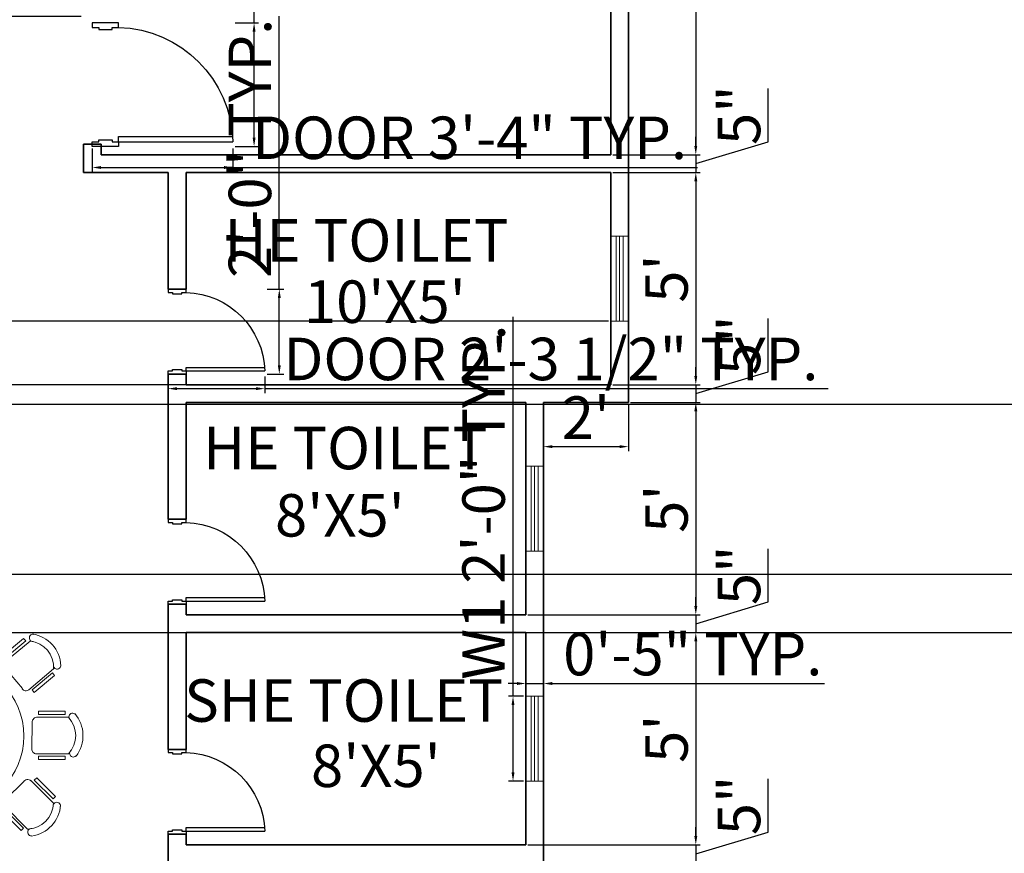
# Model space of a CAD drawing. Units: inches. Extents: x 2319 to 3765, y 2872 to 3950.
# Tile 6 of 9: x 2783 to 3061, y 3121 to 3357. Entities that reach past the tile are written whole.
import ezdxf

# ---------------------------------------------------------------- set-up
doc = ezdxf.new("R2010")
doc.units = ezdxf.units.IN
for name, color, linetype, lineweight in [('A-ANNO-DIMS', 2, 'Continuous', 18), ('A-AREA-IDEN', 7, 'Continuous', 18), ('A-DOOR', 3, 'Continuous', 25), ('A-FURN', 8, 'Continuous', 18), ('A-GLAZ', 4, 'Continuous', 18), ('A-WALL', 7, 'Continuous', 35)]:
    doc.layers.add(name, color=color, linetype=linetype, lineweight=lineweight)
doc.styles.get("Standard").update_dxf_attribs({"font": 'arial.ttf'})
doc.dimstyles.new('ISO-25', dxfattribs={"dimtxt": 12, "dimasz": 2.5, "dimexe": 1.25, "dimexo": 0.625, "dimtad": 1, "dimdec": 0, "dimlunit": 3, "dimtxsty": 'Standard', "dimcen": 2.5, "dimadec": 0, "dimazin": 0, "dimtfac": 1, "dimtdec": 0, "dimtmove": 0, "dimatfit": 3, "dimfxl": 1, "dimarcsym": 0})

# ---------------------------------------------------------------- blocks, each defined once
blk = doc.blocks.new('*D1')
at = {"layer": 'A-ANNO-DIMS', "color": 0, "lineweight": -2, "transparency": 16777216}
for p, q in [((2931.13, 3247.99), (2931.13, 3234.88)), ((2955.13, 3247.99), (2955.13, 3234.88)), ((2933.63, 3236.13), (2952.63, 3236.13))]:
    blk.add_line(p, q, dxfattribs=at)
at = {"layer": 'A-ANNO-DIMS', "color": 0, "transparency": 16777216}
for points in [[(2933.63, 3236.55), (2933.63, 3235.71), (2931.13, 3236.13)], [(2952.63, 3236.55), (2952.63, 3235.71), (2955.13, 3236.13)]]:
    blk.add_solid(points, dxfattribs=at)
at = {"layer": 'Defpoints', "color": 0, "transparency": 16777216}
for p in [(2931.13, 3248.61), (2955.13, 3248.61), (2955.13, 3236.13)]:
    blk.add_point(p, dxfattribs=at)
at = {"layer": 'A-ANNO-DIMS', "color": 0, "transparency": 16777216, "insert": (2943.13, 3242.78), "char_height": 12, "attachment_point": 5}
blk.add_mtext("2'", dxfattribs=at)
blk = doc.blocks.new('A$C769D55ED')
for p, q in [((33.6, 192), (33.6, 1024.8)), ((72, 192), (72, 1023.9)), ((0, 192), (0, 0)), ((33.6, 192), (0, 192)), ((33.6, 144), (33.6, 192)), ((48, 144), (33.6, 144)), ((48, 48), (48, 144)), ((33.6, 0), (33.6, 48)), ((33.6, 48), (48, 48)), ((0, 0), (33.6, 0))]:
    blk.add_line(p, q)
blk.add_lwpolyline([(33.6, 192), (72, 192)])
blk.add_lwpolyline([(900, 192), (900, 0), (866.4, 0), (866.4, 48), (852, 48), (852, 144), (866.4, 144), (866.4, 192)], close=True)
blk.add_arc((7.2, 165.6), 859.6, 1.76235, 88.23765)
blk = doc.blocks.new('A$C0EDB4AB9')
at = {"linetype": 'ByBlock'}
for p, q in [((1257, 3447), (1257, 3084)), ((1303, 3447), (1257, 3447)), ((1303, 3084), (1303, 3447)), ((1342, 3055), (1342, 3493)), ((1842, 3493), (1842, 3051)), ((1873, 3447), (1873, 3084)), ((1919, 3447), (1873, 3447)), ((1919, 3084), (1919, 3447)), ((2028, 3447), (2028, 3084)), ((2074, 3447), (2028, 3447)), ((2074, 3084), (2074, 3447)), ((2114, 3055), (2114, 3493)), ((2614, 3493), (2614, 3051)), ((2644, 3447), (2644, 3084)), ((2691, 3447), (2644, 3447)), ((2691, 3084), (2691, 3447)), ((2790, 3447), (2790, 3084)), ((2836, 3447), (2790, 3447)), ((2836, 3084), (2836, 3447)), ((2875, 3055), (2875, 3493)), ((3375, 3493), (3375, 3051)), ((3406, 3447), (3406, 3084)), ((3452, 3447), (3406, 3447)), ((3452, 3084), (3452, 3447)), ((3537, 3447), (3537, 3084)), ((3583, 3447), (3537, 3447)), ((3583, 3084), (3583, 3447)), ((3622, 3055), (3622, 3493)), ((4122, 3493), (4122, 3051)), ((4153, 3447), (4153, 3084)), ((4199, 3447), (4153, 3447)), ((4199, 3084), (4199, 3447)), ((4314, 3447), (4314, 3084)), ((4360, 3447), (4314, 3447)), ((4360, 3084), (4360, 3447)), ((4399, 3055), (4399, 3493)), ((4899, 3493), (4899, 3051)), ((4930, 3447), (4930, 3084)), ((4976, 3447), (4930, 3447)), ((4976, 3084), (4976, 3447)), ((5158, 3447), (5158, 3084)), ((5204, 3447), (5158, 3447)), ((5204, 3084), (5204, 3447)), ((5243, 3055), (5243, 3493)), ((5743, 3493), (5743, 3051)), ((5774, 3447), (5774, 3084)), ((5820, 3447), (5774, 3447)), ((5820, 3084), (5820, 3447)), ((5991, 3447), (5991, 3084)), ((6037, 3447), (5991, 3447)), ((6037, 3084), (6037, 3447)), ((6076, 3055), (6076, 3493)), ((6576, 3493), (6576, 3051)), ((6607, 3447), (6607, 3084)), ((6653, 3447), (6607, 3447)), ((6653, 3084), (6653, 3447)), ((770, 3117), (1098, 2820)), ((855, 3143), (824, 3109)), ((824, 3109), (1094, 2865)), ((1124, 2900), (855, 3143)), ((7050, 3209), (6772, 2975)), ((6802, 2940), (7080, 3173)), ((6804, 2891), (7139, 3172)), ((7080, 3173), (7050, 3209)), ((1257, 3084), (1303, 3084)), ((1772, 2993), (1413, 2995)), ((1791, 2993), (1772, 2993)), ((1873, 3084), (1919, 3084)), ((2028, 3084), (2074, 3084)), ((2544, 2993), (2185, 2995)), ((2562, 2993), (2544, 2993)), ((2644, 3084), (2691, 3084)), ((2790, 3084), (2836, 3084)), ((3305, 2993), (2946, 2995)), ((3324, 2993), (3305, 2993)), ((3406, 3084), (3452, 3084)), ((3537, 3084), (3583, 3084)), ((4052, 2993), (3693, 2995)), ((4070, 2993), (4052, 2993)), ((4153, 3084), (4199, 3084)), ((4314, 3084), (4360, 3084)), ((4829, 2993), (4470, 2995)), ((4847, 2993), (4829, 2993)), ((4930, 3084), (4976, 3084)), ((5158, 3084), (5204, 3084)), ((5673, 2993), (5314, 2995)), ((5692, 2993), (5673, 2993)), ((5774, 3084), (5820, 3084)), ((5991, 3084), (6037, 3084)), ((6506, 2993), (6147, 2995)), ((6525, 2993), (6506, 2993)), ((6607, 3084), (6653, 3084)), ((6772, 2975), (6802, 2940)), ((1094, 2865), (1124, 2900)), ((6056, 2871), (1856, 2871)), ((759, 2452), (435, 2746)), ((1094, 2729), (851, 2464)), ((1106, 2743), (1094, 2729)), ((7034, 2521), (6804, 2798)), ((7461, 2790), (7123, 2505)), ((7446, 2737), (7169, 2503)), ((7198, 2468), (7476, 2702)), ((7476, 2702), (7446, 2737)), ((442, 2687), (411, 2653)), ((411, 2653), (680, 2409)), ((711, 2443), (442, 2687)), ((680, 2409), (711, 2443)), ((7169, 2503), (7198, 2468)), ((608, 2159), (245, 2159)), ((245, 2159), (245, 2113)), ((608, 2113), (608, 2159)), ((7619, 2213), (7256, 2213)), ((7256, 2213), (7256, 2167)), ((7256, 2167), (7619, 2167)), ((7619, 2167), (7619, 2213)), ((200, 2082), (642, 2082)), ((245, 2113), (608, 2113)), ((700, 2031), (700, 2012)), ((7165, 1697), (7167, 2056)), ((7227, 2127), (7665, 2127)), ((700, 2012), (698, 1653)), ((7165, 1679), (7165, 1697)), ((7665, 1627), (7223, 1627)), ((638, 1582), (200, 1582)), ((608, 1543), (245, 1543)), ((245, 1543), (245, 1497)), ((245, 1497), (608, 1497)), ((608, 1497), (608, 1543)), ((7619, 1597), (7256, 1597)), ((7256, 1597), (7256, 1550)), ((7256, 1550), (7619, 1550)), ((7619, 1550), (7619, 1597)), ((748, 1304), (442, 1107)), ((446, 1018), (817, 1257)), ((467, 1068), (772, 1265)), ((772, 1265), (748, 1304)), ((894, 1245), (904, 1230)), ((904, 1230), (1097, 927)), ((6802, 1000), (7057, 1253)), ((7150, 1260), (7459, 951)), ((7231, 1300), (7198, 1267)), ((7198, 1267), (7455, 1011)), ((7487, 1043), (7231, 1300)), ((442, 1107), (467, 1068)), ((6788, 987), (6802, 1000)), ((7455, 1011), (7487, 1043)), ((1084, 834), (716, 598)), ((6056, 871), (1856, 871)), ((6795, 864), (6763, 831)), ((6763, 831), (7019, 575)), ((7106, 597), (6793, 909)), ((7052, 607), (6795, 864)), ((1081, 786), (776, 589)), ((800, 550), (1106, 747)), ((1106, 747), (1081, 786)), ((1352, 723), (1370, 723)), ((1370, 723), (1730, 722)), ((2218, 723), (2236, 723)), ((2236, 723), (2595, 722)), ((2986, 700), (3005, 700)), ((3005, 700), (3364, 698)), ((3827, 723), (3846, 723)), ((3846, 723), (4205, 722)), ((4589, 723), (4607, 723)), ((4607, 723), (4966, 722)), ((5335, 723), (5354, 723)), ((5354, 723), (5713, 722)), ((6131, 723), (6149, 723)), ((6149, 723), (6508, 722)), ((776, 589), (800, 550)), ((1270, 632), (1224, 632)), ((1224, 632), (1224, 269)), ((1270, 269), (1270, 632)), ((1300, 223), (1300, 665)), ((1800, 661), (1800, 223)), ((1886, 632), (1840, 632)), ((1840, 632), (1840, 269)), ((1886, 269), (1886, 632)), ((2135, 632), (2089, 632)), ((2089, 632), (2089, 269)), ((2135, 269), (2135, 632)), ((2166, 223), (2166, 665)), ((2666, 661), (2666, 223)), ((2752, 632), (2705, 632)), ((2705, 632), (2705, 269)), ((2752, 269), (2752, 632)), ((2904, 608), (2858, 608)), ((2858, 608), (2858, 245)), ((2904, 245), (2904, 608)), ((2935, 200), (2935, 642)), ((3435, 638), (3435, 200)), ((3520, 608), (3474, 608)), ((3474, 608), (3474, 245)), ((3520, 245), (3520, 608)), ((3745, 632), (3699, 632)), ((3699, 632), (3699, 269)), ((3745, 269), (3745, 632)), ((3776, 223), (3776, 665)), ((4276, 661), (4276, 223)), ((4361, 632), (4315, 632)), ((4315, 632), (4315, 269)), ((4361, 269), (4361, 632)), ((4507, 632), (4461, 632)), ((4461, 632), (4461, 269)), ((4507, 269), (4507, 632)), ((4537, 223), (4537, 665)), ((5037, 661), (5037, 223)), ((5123, 632), (5077, 632)), ((5077, 632), (5077, 269)), ((5123, 269), (5123, 632)), ((5253, 632), (5207, 632)), ((5207, 632), (5207, 269)), ((5253, 269), (5253, 632)), ((5284, 223), (5284, 665)), ((5784, 661), (5784, 223)), ((5869, 632), (5823, 632)), ((5823, 632), (5823, 269)), ((5869, 269), (5869, 632)), ((6049, 632), (6003, 632)), ((6003, 632), (6003, 269)), ((6049, 269), (6049, 632)), ((6079, 223), (6079, 665)), ((6579, 661), (6579, 223)), ((6665, 632), (6619, 632)), ((6619, 632), (6619, 269)), ((6665, 269), (6665, 632)), ((7019, 575), (7052, 607)), ((1224, 269), (1270, 269)), ((1840, 269), (1886, 269)), ((2089, 269), (2135, 269)), ((2705, 269), (2752, 269)), ((2858, 245), (2904, 245)), ((3474, 245), (3520, 245)), ((3699, 269), (3745, 269)), ((4315, 269), (4361, 269)), ((4461, 269), (4507, 269)), ((5077, 269), (5123, 269)), ((5207, 269), (5253, 269)), ((5823, 269), (5869, 269)), ((6003, 269), (6049, 269)), ((6619, 269), (6665, 269))]:
    blk.add_line(p, q, dxfattribs=at)
for centre, radius, start, end in [((1592, 3230), 463, 52.6032, 130.8409), ((2364, 3230), 463, 52.6032, 130.8409), ((3125, 3230), 463, 52.6032, 130.8409), ((3872, 3230), 463, 52.6032, 130.8409), ((4649, 3230), 463, 52.6032, 130.8409), ((5493, 3230), 463, 52.6032, 130.8409), ((6326, 3230), 463, 52.6032, 130.8409), ((1335, 3551), 50, 127.3845, 320.4832), ((1592, 3230), 363, 46.3972, 133.6028), ((1837, 3560), 50, 219.1941, 46.1701), ((2107, 3551), 50, 127.3845, 320.4832), ((2364, 3230), 363, 46.3972, 133.6028), ((2609, 3560), 50, 219.1941, 46.1701), ((2869, 3551), 50, 127.3845, 320.4832), ((3125, 3230), 363, 46.3972, 133.6028), ((3370, 3560), 50, 219.1941, 46.1701), ((3615, 3551), 50, 127.3845, 320.4832), ((3872, 3230), 363, 46.3972, 133.6028), ((4117, 3560), 50, 219.1941, 46.1701), ((4392, 3551), 50, 127.3845, 320.4832), ((4649, 3230), 363, 46.3972, 133.6028), ((4894, 3560), 50, 219.1941, 46.1701), ((5236, 3551), 50, 127.3845, 320.4832), ((5493, 3230), 363, 46.3972, 133.6028), ((5738, 3560), 50, 219.1941, 46.1701), ((6069, 3551), 50, 127.3845, 320.4832), ((6326, 3230), 363, 46.3972, 133.6028), ((6571, 3560), 50, 219.1941, 46.1701), ((7180, 3215), 50, 77.4483, 270.5471), ((7100, 2812), 463, 2.6671, 80.9047), ((797, 2755), 463, 100.4356, 178.6733), ((797, 2755), 363, 94.2296, 181.4352), ((717, 3158), 50, 267.0265, 94.0025), ((7100, 2812), 363, 356.461, 83.6667), ((1412, 3065), 70.2, 172.0281, 271.1673), ((1782, 3053), 60.7, 261.2421, 1.6502), ((2183, 3065), 70.2, 172.0281, 271.1673), ((2553, 3053), 60.7, 261.2421, 1.6502), ((2945, 3065), 70.2, 172.0281, 271.1673), ((3315, 3053), 60.7, 261.2421, 1.6502), ((3691, 3065), 70.2, 172.0281, 271.1673), ((4061, 3053), 60.7, 261.2421, 1.6502), ((4468, 3065), 70.2, 172.0281, 271.1673), ((4838, 3053), 60.7, 261.2421, 1.6502), ((5313, 3065), 70.2, 172.0281, 271.1673), ((5682, 3053), 60.7, 261.2421, 1.6502), ((6146, 3065), 70.2, 172.0281, 271.1673), ((6515, 3053), 60.7, 261.2421, 1.6502), ((1856, 1871), 1000, 90, 270), ((6056, 1871), 1000, 270, 90), ((6857, 2844), 70.2, 122.0919, 221.2312), ((7510, 2837), 50, 169.258, 356.234), ((386, 2780), 50, 175.2169, 8.3156), ((1056, 2776), 60.7, 309.0745, 49.4826), ((798, 2510), 70.2, 219.8605, 318.9997), ((7083, 2551), 60.7, 211.3059, 311.714), ((7723, 2134), 50, 37.3845, 230.4832), ((7402, 1877), 463, 322.6032, 40.8409), ((462, 1832), 463, 142.6032, 220.8409), ((132, 2077), 50, 309.1941, 136.1701), ((462, 1832), 363, 136.3972, 223.6028), ((640, 2021), 60.7, 351.2421, 91.6502), ((7237, 2058), 70.2, 82.0281, 181.1673), ((7402, 1877), 363, 316.3972, 43.6028), ((628, 1651), 70.2, 262.0281, 1.1673), ((7225, 1688), 60.7, 171.2421, 271.6502), ((7732, 1632), 50, 129.1941, 316.1701), ((141, 1575), 50, 217.3845, 50.4832), ((848, 1205), 60.7, 24.0035, 124.4116), ((7107, 1204), 70.2, 37.0567, 136.1959), ((802, 950), 463, 175.3647, 253.6023), ((392, 977), 50, 341.9556, 168.9315), ((802, 950), 363, 169.1586, 256.3643), ((6837, 951), 60.7, 126.2707, 226.6788), ((7097, 960), 363, 271.4258, 358.6314), ((7506, 914), 50, 352.4131, 185.5118), ((1039, 888), 70.2, 294.7895, 33.9288), ((7097, 960), 463, 277.6319, 355.8695), ((1361, 663), 60.7, 81.2421, 181.6502), ((1731, 651), 70.2, 352.0281, 91.1673), ((2227, 663), 60.7, 81.2421, 181.6502), ((2597, 651), 70.2, 352.0281, 91.1673), ((2996, 640), 60.7, 81.2421, 181.6502), ((3365, 628), 70.2, 352.0281, 91.1673), ((3836, 663), 60.7, 81.2421, 181.6502), ((4206, 651), 70.2, 352.0281, 91.1673), ((4598, 663), 60.7, 81.2421, 181.6502), ((4968, 651), 70.2, 352.0281, 91.1673), ((5345, 663), 60.7, 81.2421, 181.6502), ((5714, 651), 70.2, 352.0281, 91.1673), ((6140, 663), 60.7, 81.2421, 181.6502), ((6510, 651), 70.2, 352.0281, 91.1673), ((671, 560), 50, 250.1459, 83.2447), ((7157, 553), 50, 84.2228, 271.1987), ((1306, 156), 50, 39.1941, 226.1701), ((1550, 486), 463, 232.6032, 310.8409), ((1550, 486), 363, 226.3972, 313.6028), ((1807, 165), 50, 307.3845, 140.4832), ((2171, 156), 50, 39.1941, 226.1701), ((2416, 486), 463, 232.6032, 310.8409), ((2416, 486), 363, 226.3972, 313.6028), ((2673, 165), 50, 307.3845, 140.4832), ((2940, 132), 50, 39.1941, 226.1701), ((3185, 462), 363, 226.3972, 313.6028), ((3442, 141), 50, 307.3845, 140.4832), ((3781, 156), 50, 39.1941, 226.1701), ((4026, 486), 463, 232.6032, 310.8409), ((4026, 486), 363, 226.3972, 313.6028), ((4283, 165), 50, 307.3845, 140.4832), ((4543, 156), 50, 39.1941, 226.1701), ((4787, 486), 463, 232.6032, 310.8409), ((4787, 486), 363, 226.3972, 313.6028), ((5044, 165), 50, 307.3845, 140.4832), ((5289, 156), 50, 39.1941, 226.1701), ((5534, 486), 463, 232.6032, 310.8409), ((5534, 486), 363, 226.3972, 313.6028), ((5791, 165), 50, 307.3845, 140.4832), ((6084, 156), 50, 39.1941, 226.1701), ((6329, 486), 463, 232.6032, 310.8409), ((6329, 486), 363, 226.3972, 313.6028), ((6586, 165), 50, 307.3845, 140.4832), ((3185, 462), 463, 232.6032, 310.8409)]:
    blk.add_arc(centre, radius, start, end, dxfattribs=at)
blk = doc.blocks.new('*D8')
at = {"layer": 'A-ANNO-DIMS', "color": 0, "lineweight": -2, "transparency": 16777216}
for p, q in [((2950.75, 3438.61), (2975.43, 3438.61)), ((2974.18, 3436.11), (2974.18, 3321.11)), ((2950.75, 3318.61), (2975.43, 3318.61))]:
    blk.add_line(p, q, dxfattribs=at)
at = {"layer": 'A-ANNO-DIMS', "color": 0, "transparency": 16777216}
for points in [[(2973.76, 3436.11), (2974.59, 3436.11), (2974.18, 3438.61)], [(2973.76, 3321.11), (2974.59, 3321.11), (2974.18, 3318.61)]]:
    blk.add_solid(points, dxfattribs=at)
at = {"layer": 'Defpoints', "color": 0, "transparency": 16777216}
for p in [(2950.13, 3438.61), (2950.13, 3318.61), (2974.18, 3318.61)]:
    blk.add_point(p, dxfattribs=at)
at = {"layer": 'A-ANNO-DIMS', "color": 0, "transparency": 16777216, "insert": (2967.42, 3378.61), "char_height": 12, "attachment_point": 5, "rotation": 90}
blk.add_mtext("10'", dxfattribs=at)
blk = doc.blocks.new('*D9')
at = {"layer": 'A-ANNO-DIMS', "color": 0, "lineweight": -2, "transparency": 16777216}
for p, q in [((2994.67, 3322.26), (2994.67, 3337.3)), ((2974.18, 3321.11), (2974.18, 3323.61)), ((2974.18, 3316.11), (2994.67, 3322.26)), ((2950.75, 3318.61), (2975.43, 3318.61)), ((2974.18, 3318.61), (2974.18, 3313.61)), ((2974.18, 3318.61), (2974.18, 3313.61)), ((2950.75, 3313.61), (2975.43, 3313.61)), ((2974.18, 3311.11), (2974.18, 3308.61))]:
    blk.add_line(p, q, dxfattribs=at)
at = {"layer": 'A-ANNO-DIMS', "color": 0, "transparency": 16777216}
for points in [[(2973.76, 3321.11), (2974.59, 3321.11), (2974.18, 3318.61)], [(2973.76, 3311.11), (2974.59, 3311.11), (2974.18, 3313.61)]]:
    blk.add_solid(points, dxfattribs=at)
at = {"layer": 'Defpoints', "color": 0, "transparency": 16777216}
for p in [(2950.13, 3318.61), (2950.13, 3313.61), (2974.18, 3313.61)]:
    blk.add_point(p, dxfattribs=at)
at = {"layer": 'A-ANNO-DIMS', "color": 0, "transparency": 16777216, "insert": (2987.94, 3329.78), "char_height": 12, "attachment_point": 5, "rotation": 90}
blk.add_mtext('5"', dxfattribs=at)
blk = doc.blocks.new('*D10')
at = {"layer": 'A-ANNO-DIMS', "color": 0, "lineweight": -2, "transparency": 16777216}
for p, q in [((2950.75, 3313.61), (2975.43, 3313.61)), ((2974.18, 3311.11), (2974.18, 3256.11)), ((2950.75, 3253.61), (2975.43, 3253.61))]:
    blk.add_line(p, q, dxfattribs=at)
at = {"layer": 'A-ANNO-DIMS', "color": 0, "transparency": 16777216}
for points in [[(2973.76, 3311.11), (2974.59, 3311.11), (2974.18, 3313.61)], [(2973.76, 3256.11), (2974.59, 3256.11), (2974.18, 3253.61)]]:
    blk.add_solid(points, dxfattribs=at)
at = {"layer": 'Defpoints', "color": 0, "transparency": 16777216}
for p in [(2950.13, 3313.61), (2950.13, 3253.61), (2974.18, 3253.61)]:
    blk.add_point(p, dxfattribs=at)
at = {"layer": 'A-ANNO-DIMS', "color": 0, "transparency": 16777216, "insert": (2967.45, 3283.61), "char_height": 12, "attachment_point": 5, "rotation": 90}
blk.add_mtext("5'", dxfattribs=at)
blk = doc.blocks.new('*D11')
at = {"layer": 'A-ANNO-DIMS', "color": 0, "lineweight": -2, "transparency": 16777216}
for p, q in [((2994.67, 3257.26), (2994.67, 3272.3)), ((2974.18, 3256.11), (2974.18, 3258.61)), ((2974.18, 3251.11), (2994.67, 3257.26)), ((2950.75, 3253.61), (2975.43, 3253.61)), ((2974.18, 3253.61), (2974.18, 3248.61)), ((2974.18, 3253.61), (2974.18, 3248.61)), ((2955.75, 3248.61), (2975.43, 3248.61)), ((2974.18, 3246.11), (2974.18, 3243.61))]:
    blk.add_line(p, q, dxfattribs=at)
at = {"layer": 'A-ANNO-DIMS', "color": 0, "transparency": 16777216}
for points in [[(2973.76, 3256.11), (2974.59, 3256.11), (2974.18, 3253.61)], [(2973.76, 3246.11), (2974.59, 3246.11), (2974.18, 3248.61)]]:
    blk.add_solid(points, dxfattribs=at)
at = {"layer": 'Defpoints', "color": 0, "transparency": 16777216}
for p in [(2950.13, 3253.61), (2955.13, 3248.61), (2974.18, 3248.61)]:
    blk.add_point(p, dxfattribs=at)
at = {"layer": 'A-ANNO-DIMS', "color": 0, "transparency": 16777216, "insert": (2987.94, 3264.78), "char_height": 12, "attachment_point": 5, "rotation": 90}
blk.add_mtext('5"', dxfattribs=at)
blk = doc.blocks.new('*D12')
at = {"layer": 'A-ANNO-DIMS', "color": 0, "lineweight": -2, "transparency": 16777216}
for p, q in [((2955.75, 3248.61), (2975.43, 3248.61)), ((2974.18, 3246.11), (2974.18, 3191.11)), ((2926.75, 3188.61), (2975.43, 3188.61))]:
    blk.add_line(p, q, dxfattribs=at)
at = {"layer": 'A-ANNO-DIMS', "color": 0, "transparency": 16777216}
for points in [[(2973.76, 3246.11), (2974.59, 3246.11), (2974.18, 3248.61)], [(2973.76, 3191.11), (2974.59, 3191.11), (2974.18, 3188.61)]]:
    blk.add_solid(points, dxfattribs=at)
at = {"layer": 'Defpoints', "color": 0, "transparency": 16777216}
for p in [(2955.13, 3248.61), (2926.13, 3188.61), (2974.18, 3188.61)]:
    blk.add_point(p, dxfattribs=at)
at = {"layer": 'A-ANNO-DIMS', "color": 0, "transparency": 16777216, "insert": (2967.45, 3218.61), "char_height": 12, "attachment_point": 5, "rotation": 90}
blk.add_mtext("5'", dxfattribs=at)
blk = doc.blocks.new('*D13')
at = {"layer": 'A-ANNO-DIMS', "color": 0, "lineweight": -2, "transparency": 16777216}
for p, q in [((2994.67, 3192.26), (2994.67, 3207.3)), ((2974.18, 3191.11), (2974.18, 3193.61)), ((2974.18, 3186.11), (2994.67, 3192.26)), ((2926.75, 3188.61), (2975.43, 3188.61)), ((2974.18, 3188.61), (2974.18, 3183.61)), ((2974.18, 3188.61), (2974.18, 3183.61)), ((2926.75, 3183.61), (2975.43, 3183.61)), ((2974.18, 3181.11), (2974.18, 3178.61))]:
    blk.add_line(p, q, dxfattribs=at)
at = {"layer": 'A-ANNO-DIMS', "color": 0, "transparency": 16777216}
for points in [[(2973.76, 3191.11), (2974.59, 3191.11), (2974.18, 3188.61)], [(2973.76, 3181.11), (2974.59, 3181.11), (2974.18, 3183.61)]]:
    blk.add_solid(points, dxfattribs=at)
at = {"layer": 'Defpoints', "color": 0, "transparency": 16777216}
for p in [(2926.13, 3188.61), (2926.13, 3183.61), (2974.18, 3183.61)]:
    blk.add_point(p, dxfattribs=at)
at = {"layer": 'A-ANNO-DIMS', "color": 0, "transparency": 16777216, "insert": (2987.94, 3199.78), "char_height": 12, "attachment_point": 5, "rotation": 90}
blk.add_mtext('5"', dxfattribs=at)
blk = doc.blocks.new('*D14')
at = {"layer": 'A-ANNO-DIMS', "color": 0, "lineweight": -2, "transparency": 16777216}
for p, q in [((2926.75, 3183.61), (2975.43, 3183.61)), ((2974.18, 3181.11), (2974.18, 3126.11)), ((2926.75, 3123.61), (2975.43, 3123.61))]:
    blk.add_line(p, q, dxfattribs=at)
at = {"layer": 'A-ANNO-DIMS', "color": 0, "transparency": 16777216}
for points in [[(2973.76, 3181.11), (2974.59, 3181.11), (2974.18, 3183.61)], [(2973.76, 3126.11), (2974.59, 3126.11), (2974.18, 3123.61)]]:
    blk.add_solid(points, dxfattribs=at)
at = {"layer": 'Defpoints', "color": 0, "transparency": 16777216}
for p in [(2926.13, 3183.61), (2926.13, 3123.61), (2974.18, 3123.61)]:
    blk.add_point(p, dxfattribs=at)
at = {"layer": 'A-ANNO-DIMS', "color": 0, "transparency": 16777216, "insert": (2967.45, 3153.61), "char_height": 12, "attachment_point": 5, "rotation": 90}
blk.add_mtext("5'", dxfattribs=at)
blk = doc.blocks.new('*D15')
at = {"layer": 'A-ANNO-DIMS', "color": 0, "lineweight": -2, "transparency": 16777216}
for p, q in [((2994.67, 3127.26), (2994.67, 3142.3)), ((2974.18, 3126.11), (2974.18, 3128.61)), ((2974.18, 3121.11), (2994.67, 3127.26)), ((2926.75, 3123.61), (2975.43, 3123.61)), ((2974.18, 3123.61), (2974.18, 3118.61)), ((2974.18, 3123.61), (2974.18, 3118.61)), ((2926.75, 3118.61), (2975.43, 3118.61)), ((2974.18, 3116.11), (2974.18, 3113.61))]:
    blk.add_line(p, q, dxfattribs=at)
at = {"layer": 'A-ANNO-DIMS', "color": 0, "transparency": 16777216}
for points in [[(2973.76, 3126.11), (2974.59, 3126.11), (2974.18, 3123.61)], [(2973.76, 3116.11), (2974.59, 3116.11), (2974.18, 3118.61)]]:
    blk.add_solid(points, dxfattribs=at)
at = {"layer": 'Defpoints', "color": 0, "transparency": 16777216}
for p in [(2926.13, 3123.61), (2926.13, 3118.61), (2974.18, 3118.61)]:
    blk.add_point(p, dxfattribs=at)
at = {"layer": 'A-ANNO-DIMS', "color": 0, "transparency": 16777216, "insert": (2987.94, 3134.78), "char_height": 12, "attachment_point": 5, "rotation": 90}
blk.add_mtext('5"', dxfattribs=at)
blk = doc.blocks.new('WIN-24-PLAN-5IN-WALL')
for p, q in [((0, 24), (5, 24)), ((1.5, 0), (1.5, 24)), ((2.5, 0), (2.5, 24)), ((3.5, 0), (3.5, 24)), ((0, 0), (5, 0))]:
    blk.add_line(p, q)
blk = doc.blocks.new('*D45')
at = {"layer": 'A-ANNO-DIMS', "color": 0, "lineweight": -2, "transparency": 16777216}
for p, q in [((2825.07, 3255.99), (2825.07, 3251.26)), ((2852.39, 3255.99), (2852.39, 3251.26)), ((2827.57, 3252.51), (2849.89, 3252.51)), ((2852.39, 3252.51), (3011.6, 3252.51))]:
    blk.add_line(p, q, dxfattribs=at)
at = {"layer": 'A-ANNO-DIMS', "color": 0, "transparency": 16777216}
for points in [[(2827.57, 3252.93), (2827.57, 3252.1), (2825.07, 3252.51)], [(2849.89, 3252.93), (2849.89, 3252.1), (2852.39, 3252.51)]]:
    blk.add_solid(points, dxfattribs=at)
at = {"layer": 'Defpoints', "color": 0, "transparency": 16777216}
for p in [(2825.07, 3256.61), (2852.39, 3256.61), (2852.39, 3252.51)]:
    blk.add_point(p, dxfattribs=at)
at = {"layer": 'A-ANNO-DIMS', "color": 0, "transparency": 16777216, "insert": (2933.25, 3259.35), "char_height": 12, "attachment_point": 5}
blk.add_mtext('DOOR 2\'-3 1/2" TYP.', dxfattribs=at)
blk = doc.blocks.new('*D46')
at = {"layer": 'A-ANNO-DIMS', "color": 0, "lineweight": -2, "transparency": 16777216}
for p, q in [((2856.49, 3280.61), (2856.49, 3357.71)), ((2853.02, 3280.61), (2857.74, 3280.61)), ((2856.49, 3259.11), (2856.49, 3278.11)), ((2853.02, 3256.61), (2857.74, 3256.61))]:
    blk.add_line(p, q, dxfattribs=at)
at = {"layer": 'A-ANNO-DIMS', "color": 0, "transparency": 16777216}
for points in [[(2856.07, 3278.11), (2856.91, 3278.11), (2856.49, 3280.61)], [(2856.07, 3259.11), (2856.91, 3259.11), (2856.49, 3256.61)]]:
    blk.add_solid(points, dxfattribs=at)
at = {"layer": 'Defpoints', "color": 0, "transparency": 16777216}
for p in [(2852.39, 3280.61), (2856.49, 3280.61), (2852.39, 3256.61)]:
    blk.add_point(p, dxfattribs=at)
at = {"layer": 'A-ANNO-DIMS', "color": 0, "transparency": 16777216, "insert": (2849.74, 3320.41), "char_height": 12, "attachment_point": 5, "rotation": 90}
blk.add_mtext('2\'-0" TYP.', dxfattribs=at)
blk = doc.blocks.new('*D47')
at = {"layer": 'A-ANNO-DIMS', "color": 0, "lineweight": -2, "transparency": 16777216}
for p, q in [((2803.63, 3320.33), (2803.63, 3313.74)), ((2843.4, 3320.33), (2843.4, 3313.74)), ((2806.13, 3314.99), (2840.9, 3314.99)), ((2843.4, 3314.99), (2974.65, 3314.99))]:
    blk.add_line(p, q, dxfattribs=at)
at = {"layer": 'A-ANNO-DIMS', "color": 0, "transparency": 16777216}
for points in [[(2806.13, 3315.41), (2806.13, 3314.58), (2803.63, 3314.99)], [(2840.9, 3315.41), (2840.9, 3314.58), (2843.4, 3314.99)]]:
    blk.add_solid(points, dxfattribs=at)
at = {"layer": 'Defpoints', "color": 0, "transparency": 16777216}
for p in [(2803.63, 3320.96), (2843.4, 3320.96), (2843.4, 3314.99)]:
    blk.add_point(p, dxfattribs=at)
at = {"layer": 'A-ANNO-DIMS', "color": 0, "transparency": 16777216, "insert": (2910.27, 3321.83), "char_height": 12, "attachment_point": 5}
blk.add_mtext('DOOR 3\'-4" TYP.', dxfattribs=at)
blk = doc.blocks.new('*D48')
at = {"layer": 'A-ANNO-DIMS', "color": 0, "lineweight": -2, "transparency": 16777216}
for p, q in [((2849.36, 3355.89), (2849.36, 3442.31)), ((2844.02, 3355.89), (2850.61, 3355.89)), ((2849.36, 3323.46), (2849.36, 3353.39)), ((2844.02, 3320.96), (2850.61, 3320.96))]:
    blk.add_line(p, q, dxfattribs=at)
at = {"layer": 'A-ANNO-DIMS', "color": 0, "transparency": 16777216}
for points in [[(2848.95, 3353.39), (2849.78, 3353.39), (2849.36, 3355.89)], [(2848.95, 3323.46), (2849.78, 3323.46), (2849.36, 3320.96)]]:
    blk.add_solid(points, dxfattribs=at)
at = {"layer": 'Defpoints', "color": 0, "transparency": 16777216}
for p in [(2843.4, 3355.89), (2849.36, 3355.89), (2843.4, 3320.96)]:
    blk.add_point(p, dxfattribs=at)
at = {"layer": 'A-ANNO-DIMS', "color": 0, "transparency": 16777216, "insert": (2842.71, 3400.35), "char_height": 12, "attachment_point": 5, "rotation": 90}
blk.add_mtext('2\'-11" TYP.', dxfattribs=at)
blk = doc.blocks.new('*D57')
at = {"layer": 'A-ANNO-DIMS', "color": 0, "lineweight": -2, "transparency": 16777216}
for p, q in [((2922.53, 3165.61), (2922.53, 3272.8)), ((2925.5, 3165.61), (2921.28, 3165.61)), ((2922.53, 3144.11), (2922.53, 3163.11)), ((2925.5, 3141.61), (2921.28, 3141.61))]:
    blk.add_line(p, q, dxfattribs=at)
at = {"layer": 'A-ANNO-DIMS', "color": 0, "transparency": 16777216}
for points in [[(2922.11, 3163.11), (2922.94, 3163.11), (2922.53, 3165.61)], [(2922.11, 3144.11), (2922.94, 3144.11), (2922.53, 3141.61)]]:
    blk.add_solid(points, dxfattribs=at)
at = {"layer": 'Defpoints', "color": 0, "transparency": 16777216}
for p in [(2922.53, 3165.61), (2926.13, 3165.61), (2926.13, 3141.61)]:
    blk.add_point(p, dxfattribs=at)
at = {"layer": 'A-ANNO-DIMS', "color": 0, "transparency": 16777216, "insert": (2915.77, 3220.46), "char_height": 12, "attachment_point": 5, "rotation": 90}
blk.add_mtext('W1 2\'-0" TYP.', dxfattribs=at)
blk = doc.blocks.new('*D58')
at = {"layer": 'A-ANNO-DIMS', "color": 0, "lineweight": -2, "transparency": 16777216}
for p, q in [((2923.63, 3169.21), (2921.13, 3169.21)), ((2926.13, 3166.24), (2926.13, 3170.46)), ((2926.13, 3169.21), (2931.13, 3169.21)), ((2931.13, 3166.24), (2931.13, 3170.46)), ((2933.63, 3169.21), (3010.52, 3169.21))]:
    blk.add_line(p, q, dxfattribs=at)
at = {"layer": 'A-ANNO-DIMS', "color": 0, "transparency": 16777216}
for points in [[(2923.63, 3169.63), (2923.63, 3168.79), (2926.13, 3169.21)], [(2933.63, 3169.63), (2933.63, 3168.79), (2931.13, 3169.21)]]:
    blk.add_solid(points, dxfattribs=at)
at = {"layer": 'Defpoints', "color": 0, "transparency": 16777216}
for p in [(2931.13, 3169.21), (2926.13, 3165.61), (2931.13, 3165.61)]:
    blk.add_point(p, dxfattribs=at)
at = {"layer": 'A-ANNO-DIMS', "color": 0, "transparency": 16777216, "insert": (2973.32, 3175.96), "char_height": 12, "attachment_point": 5}
blk.add_mtext('0\'-5" TYP.', dxfattribs=at)
blk = doc.blocks.new('*D72')
at = {"layer": 'A-ANNO-DIMS', "color": 0, "lineweight": -2, "transparency": 16777216}
for p, q in [((2955.75, 3568.61), (3085.2, 3568.61)), ((3083.95, 2963.11), (3083.95, 3566.11)), ((2955.75, 2960.61), (3085.2, 2960.61))]:
    blk.add_line(p, q, dxfattribs=at)
at = {"layer": 'A-ANNO-DIMS', "color": 0, "transparency": 16777216}
for points in [[(3083.53, 3566.11), (3084.36, 3566.11), (3083.95, 3568.61)], [(3083.53, 2963.11), (3084.36, 2963.11), (3083.95, 2960.61)]]:
    blk.add_solid(points, dxfattribs=at)
at = {"layer": 'Defpoints', "color": 0, "transparency": 16777216}
for p in [(2955.13, 3568.61), (3083.95, 3568.61), (2955.13, 2960.61)]:
    blk.add_point(p, dxfattribs=at)
at = {"layer": 'A-ANNO-DIMS', "color": 0, "transparency": 16777216, "insert": (3077.2, 3264.61), "char_height": 12, "attachment_point": 5, "rotation": 90}
blk.add_mtext('50\'-8"', dxfattribs=at)
blk = doc.blocks.new('*D76')
at = {"layer": 'A-ANNO-DIMS', "color": 0, "lineweight": -2, "transparency": 16777216}
for p, q in [((2757.13, 2970.24), (2757.13, 3605.01)), ((2759.63, 3603.76), (2773.17, 3603.76)), ((2775.67, 2970.24), (2775.67, 3605.01)), ((2775.67, 3603.76), (2838.15, 3603.76))]:
    blk.add_line(p, q, dxfattribs=at)
at = {"layer": 'A-ANNO-DIMS', "color": 0, "transparency": 16777216}
for points in [[(2759.63, 3604.18), (2759.63, 3603.34), (2757.13, 3603.76)], [(2773.17, 3604.18), (2773.17, 3603.34), (2775.67, 3603.76)]]:
    blk.add_solid(points, dxfattribs=at)
at = {"layer": 'Defpoints', "color": 0, "transparency": 16777216}
for p in [(2775.67, 3603.76), (2757.13, 2969.61), (2775.67, 2969.61)]:
    blk.add_point(p, dxfattribs=at)
at = {"layer": 'A-ANNO-DIMS', "color": 0, "transparency": 16777216, "insert": (2808.16, 3610.59), "char_height": 12, "attachment_point": 5}
blk.add_mtext('1\'-6 1/2"', dxfattribs=at)
blk = doc.blocks.new('*D81')
at = {"layer": 'A-ANNO-DIMS', "color": 0, "lineweight": -2, "transparency": 16777216}
for p, q in [((2603.75, 3248.11), (3085.2, 3248.11)), ((3083.95, 3202.61), (3083.95, 3245.61)), ((2603.75, 3200.11), (3085.2, 3200.11))]:
    blk.add_line(p, q, dxfattribs=at)
at = {"layer": 'A-ANNO-DIMS', "color": 0, "transparency": 16777216}
for points in [[(3083.53, 3245.61), (3084.36, 3245.61), (3083.95, 3248.11)], [(3083.53, 3202.61), (3084.36, 3202.61), (3083.95, 3200.11)]]:
    blk.add_solid(points, dxfattribs=at)
at = {"layer": 'Defpoints', "color": 0, "transparency": 16777216}
for p in [(2603.13, 3248.11), (3083.95, 3248.11), (2603.13, 3200.11)]:
    blk.add_point(p, dxfattribs=at)
at = {"layer": 'A-ANNO-DIMS', "color": 0, "transparency": 16777216, "insert": (3077.2, 3224.11), "char_height": 12, "attachment_point": 5, "rotation": 90}
blk.add_mtext('4\'-0"', dxfattribs=at)
blk = doc.blocks.new('*D82')
at = {"layer": 'A-ANNO-DIMS', "color": 0, "lineweight": -2, "transparency": 16777216}
for p, q in [((3083.95, 3200.11), (3083.95, 3262.59)), ((2603.75, 3200.11), (3085.2, 3200.11)), ((3083.95, 3186.11), (3083.95, 3197.61)), ((2603.75, 3183.61), (3085.2, 3183.61))]:
    blk.add_line(p, q, dxfattribs=at)
at = {"layer": 'A-ANNO-DIMS', "color": 0, "transparency": 16777216}
for points in [[(3083.53, 3197.61), (3084.36, 3197.61), (3083.95, 3200.11)], [(3083.53, 3186.11), (3084.36, 3186.11), (3083.95, 3183.61)]]:
    blk.add_solid(points, dxfattribs=at)
at = {"layer": 'Defpoints', "color": 0, "transparency": 16777216}
for p in [(2603.13, 3200.11), (3083.95, 3200.11), (2603.13, 3183.61)]:
    blk.add_point(p, dxfattribs=at)
at = {"layer": 'A-ANNO-DIMS', "color": 0, "transparency": 16777216, "insert": (3077.12, 3232.6), "char_height": 12, "attachment_point": 5, "rotation": 90}
blk.add_mtext('1\'-4 1/2"', dxfattribs=at)
blk = doc.blocks.new('*D87')
at = {"layer": 'A-ANNO-DIMS', "color": 0, "lineweight": -2, "transparency": 16777216}
for p, q in [((2800.5, 3380.11), (2341.89, 3380.11)), ((2343.14, 3377.61), (2343.14, 3360.11)), ((2800.5, 3357.61), (2341.89, 3357.61)), ((2343.14, 3357.61), (2343.14, 3285.81))]:
    blk.add_line(p, q, dxfattribs=at)
at = {"layer": 'A-ANNO-DIMS', "color": 0, "transparency": 16777216}
for points in [[(2342.72, 3377.61), (2343.56, 3377.61), (2343.14, 3380.11)], [(2342.72, 3360.11), (2343.56, 3360.11), (2343.14, 3357.61)]]:
    blk.add_solid(points, dxfattribs=at)
at = {"layer": 'Defpoints', "color": 0, "transparency": 16777216}
for p in [(2801.13, 3380.11), (2343.14, 3357.61), (2801.13, 3357.61)]:
    blk.add_point(p, dxfattribs=at)
at = {"layer": 'A-ANNO-DIMS', "color": 0, "transparency": 16777216, "insert": (2336.31, 3320.46), "char_height": 12, "attachment_point": 5, "rotation": 90}
blk.add_mtext('1\'-10 1/2"', dxfattribs=at)
blk = doc.blocks.new('*D88')
at = {"layer": 'A-ANNO-DIMS', "color": 0, "lineweight": -2, "transparency": 16777216}
for p, q in [((2343.14, 3271.61), (2343.14, 3306.13)), ((2949.5, 3271.61), (2341.89, 3271.61)), ((2343.14, 3256.11), (2343.14, 3269.11)), ((2949.5, 3253.61), (2341.89, 3253.61))]:
    blk.add_line(p, q, dxfattribs=at)
at = {"layer": 'A-ANNO-DIMS', "color": 0, "transparency": 16777216}
for points in [[(2342.72, 3269.11), (2343.56, 3269.11), (2343.14, 3271.61)], [(2342.72, 3256.11), (2343.56, 3256.11), (2343.14, 3253.61)]]:
    blk.add_solid(points, dxfattribs=at)
at = {"layer": 'Defpoints', "color": 0, "transparency": 16777216}
for p in [(2343.14, 3271.61), (2950.13, 3271.61), (2950.13, 3253.61)]:
    blk.add_point(p, dxfattribs=at)
at = {"layer": 'A-ANNO-DIMS', "color": 0, "transparency": 16777216, "insert": (2336.39, 3290.12), "char_height": 12, "attachment_point": 5, "rotation": 90}
blk.add_mtext('1\'-6"', dxfattribs=at)

msp = doc.modelspace()

# ---------------------------------------------------------------- linework, layer by layer
at = {"layer": 'A-GLAZ'}
for p, q in [((2927.63, 3206.61), (2927.63, 3230.61)), ((2926.13, 3165.61), (2931.13, 3165.61))]:
    msp.add_line(p, q, dxfattribs=at)
at = {"layer": 'A-WALL'}
for p, q in [((2955.13, 3248.61), (2955.13, 3443.61)), ((2950.13, 3318.61), (2950.13, 3438.61)), ((2806.13, 3321.61), (2801.13, 3321.61)), ((2801.13, 3321.61), (2801.13, 3313.61)), ((2806.13, 3321.61), (2806.13, 3318.61)), ((2950.13, 3318.61), (2806.13, 3318.61)), ((2825.13, 3313.61), (2801.13, 3313.61)), ((2825.13, 3280.61), (2825.13, 3313.61)), ((2950.13, 3313.61), (2830.13, 3313.61)), ((2830.13, 3280.61), (2830.13, 3313.61)), ((2950.13, 3253.61), (2950.13, 3313.61)), ((2830.13, 3280.61), (2825.13, 3280.61)), ((2825.13, 3215.61), (2825.13, 3256.61)), ((2830.13, 3256.61), (2825.13, 3256.61)), ((2830.13, 3253.61), (2830.13, 3256.61)), ((2931.13, 3253.61), (2830.13, 3253.61)), ((2830.13, 3253.61), (2950.13, 3253.61)), ((2926.13, 3248.61), (2830.13, 3248.61)), ((2830.13, 3215.61), (2830.13, 3248.61)), ((2926.13, 3188.61), (2926.13, 3248.61)), ((2931.13, 3058.61), (2931.13, 3248.61)), ((2931.13, 3248.61), (2955.13, 3248.61)), ((2830.13, 3215.61), (2825.13, 3215.61)), ((2825.13, 3150.61), (2825.13, 3191.61)), ((2830.13, 3191.61), (2825.13, 3191.61)), ((2830.13, 3188.61), (2830.13, 3191.61)), ((2926.13, 3188.61), (2830.13, 3188.61)), ((2926.13, 3183.61), (2830.13, 3183.61)), ((2830.13, 3150.61), (2830.13, 3183.61)), ((2926.13, 3123.61), (2926.13, 3183.61)), ((2830.13, 3150.61), (2825.13, 3150.61)), ((2825.13, 3085.61), (2825.13, 3126.61)), ((2830.13, 3126.61), (2825.13, 3126.61)), ((2830.13, 3123.61), (2830.13, 3126.61)), ((2926.13, 3123.61), (2830.13, 3123.61))]:
    msp.add_line(p, q, dxfattribs=at)

# ---------------------------------------------------------------- block references
at = {"layer": 'A-DOOR', "rotation": 270}
for p, xscale, yscale, zscale in [((2803.63, 3320.96), -0.0388089662083284, 0.0388089662083284, 0.0388089662083284), ((2825.07, 3256.61), -0.0266624880085475, 0.0266624880085475, 0.0266624880085475), ((2825.07, 3191.61), -0.0266624880085475, 0.0266624880085475, 0.0266624880085475), ((2825.07, 3126.61), -0.0266624880085475, 0.0266624880085475, 0.0266624880085475)]:
    msp.add_blockref('A$C769D55ED', p, dxfattribs=dict(at, xscale=xscale, yscale=yscale, zscale=zscale))
at = {"layer": 'A-FURN', "xscale": 0.02062408179219, "yscale": 0.02062408179219, "zscale": 0.02062408179219}
msp.add_blockref('A$C0EDB4AB9', (2638.81, 3115.79), dxfattribs=at)
at = {"layer": 'A-GLAZ'}
for p in [(2950.13, 3271.61), (2926.13, 3206.61), (2926.13, 3141.61)]:
    msp.add_blockref('WIN-24-PLAN-5IN-WALL', p, dxfattribs=at)

# ---------------------------------------------------------------- texts
at = {"layer": 'A-AREA-IDEN'}
for s, p in [('HE TOILET', (2840.97, 3288.41)), ("10'X5'", (2863.46, 3271.08)), ('HE TOILET', (2834.96, 3229.73)), ("8'X5'", (2855.29, 3210.73)), ('SHE TOILET', (2829.63, 3158.4)), ("8'X5'", (2865.46, 3139.97))]:
    msp.add_text(s, height=12, dxfattribs=at).set_placement(p)

# ---------------------------------------------------------------- dimensions: what is measured, and where the dimension line sits
at = {"layer": 'A-ANNO-DIMS'}
for base, p1, p2, override, picture, middle in [((2775.67, 3603.76), (2757.13, 2969.61), (2775.67, 2969.61), {"dimdec": 1, "dimlfac": 1, "dimrnd": 0, "dimzin": 1, "dimdsep": 46, "dimlunit": 4, "dimfrac": 2}, '*D76', (2808.16, 3610.59)), ((2955.13, 3236.13), (2931.13, 3248.61), (2955.13, 3248.61), {"dimclrd": 0, "dimclre": 0, "dimclrt": 0}, '*D1', (2943.13, 3242.78))]:
    dim = msp.add_linear_dim(base=base, p1=p1, p2=p2, dimstyle='ISO-25', override=override, dxfattribs=at)
    dim.commit()
    dim.dimension.update_dxf_attribs({"geometry": picture, "text_midpoint": middle})
for base, p1, p2, override, picture, middle in [((3083.95, 3568.61), (2955.13, 2960.61), (2955.13, 3568.61), {"dimdec": 1, "dimlfac": 1, "dimrnd": 0, "dimzin": 1, "dimdsep": 46, "dimlunit": 4, "dimfrac": 2}, '*D72', (3077.2, 3264.61)), ((2974.18, 3318.61), (2950.13, 3438.61), (2950.13, 3318.61), {"dimclrd": 0, "dimclre": 0, "dimclrt": 0, "dimtmove": 1}, '*D8', (2967.42, 3378.61)), ((2343.14, 3357.61), (2801.13, 3380.11), (2801.13, 3357.61), {"dimdec": 1, "dimlfac": 1, "dimrnd": 0, "dimzin": 1, "dimdsep": 46, "dimlunit": 4, "dimfrac": 2}, '*D87', (2336.31, 3320.46)), ((2974.18, 3313.61), (2950.13, 3318.61), (2950.13, 3313.61), {"dimclrd": 0, "dimclre": 0, "dimclrt": 0, "dimtmove": 1}, '*D9', (2987.94, 3322.88)), ((2974.18, 3253.61), (2950.13, 3313.61), (2950.13, 3253.61), {"dimclrd": 0, "dimclre": 0, "dimclrt": 0, "dimtmove": 1}, '*D10', (2967.45, 3283.61)), ((2343.14, 3271.61), (2950.13, 3253.61), (2950.13, 3271.61), {"dimdec": 1, "dimlfac": 1, "dimrnd": 0, "dimzin": 1, "dimdsep": 46, "dimlunit": 4, "dimfrac": 2}, '*D88', (2336.39, 3290.12)), ((2974.18, 3248.61), (2950.13, 3253.61), (2955.13, 3248.61), {"dimclrd": 0, "dimclre": 0, "dimclrt": 0, "dimtmove": 1}, '*D11', (2987.94, 3257.88)), ((3083.95, 3200.11), (2603.13, 3183.61), (2603.13, 3200.11), {"dimdec": 1, "dimlfac": 1, "dimrnd": 0, "dimzin": 1, "dimdsep": 46, "dimlunit": 4, "dimfrac": 2}, '*D82', (3077.12, 3232.6)), ((3083.95, 3248.11), (2603.13, 3200.11), (2603.13, 3248.11), {"dimdec": 1, "dimlfac": 1, "dimrnd": 0, "dimzin": 1, "dimdsep": 46, "dimlunit": 4, "dimfrac": 2}, '*D81', (3077.2, 3224.11)), ((2974.18, 3188.61), (2955.13, 3248.61), (2926.13, 3188.61), {"dimclrd": 0, "dimclre": 0, "dimclrt": 0, "dimtmove": 1}, '*D12', (2967.45, 3218.61)), ((2974.18, 3183.61), (2926.13, 3188.61), (2926.13, 3183.61), {"dimclrd": 0, "dimclre": 0, "dimclrt": 0, "dimtmove": 1}, '*D13', (2987.94, 3192.88)), ((2974.18, 3123.61), (2926.13, 3183.61), (2926.13, 3123.61), {"dimclrd": 0, "dimclre": 0, "dimclrt": 0, "dimtmove": 1}, '*D14', (2967.45, 3153.61)), ((2974.18, 3118.61), (2926.13, 3123.61), (2926.13, 3118.61), {"dimclrd": 0, "dimclre": 0, "dimclrt": 0, "dimtmove": 1}, '*D15', (2987.94, 3127.88))]:
    dim = msp.add_linear_dim(base=base, p1=p1, p2=p2, angle=90, dimstyle='ISO-25', override=override, dxfattribs=at)
    dim.commit()
    dim.dimension.update_dxf_attribs({"geometry": picture, "text_midpoint": middle})
for base, p1, p2, text, picture, middle in [((2849.36, 3355.89), (2843.4, 3320.96), (2843.4, 3355.89), '<> TYP.', '*D48', (2842.71, 3400.35)), ((2856.49, 3280.61), (2852.39, 3256.61), (2852.39, 3280.61), '<> TYP.', '*D46', (2849.74, 3320.41)), ((2922.53, 3165.61), (2926.13, 3141.61), (2926.13, 3165.61), 'W1 <> TYP.', '*D57', (2915.77, 3220.46))]:
    dim = msp.add_linear_dim(base=base, p1=p1, p2=p2, angle=90, text=text, dimstyle='ISO-25', override={"dimdec": 1, "dimlfac": 1, "dimrnd": 0, "dimzin": 1, "dimdsep": 46, "dimlunit": 4, "dimfrac": 2}, dxfattribs=at)
    dim.commit()
    dim.dimension.update_dxf_attribs({"geometry": picture, "text_midpoint": middle})
for base, p1, p2, text, picture, middle in [((2843.4, 3314.99), (2803.63, 3320.96), (2843.4, 3320.96), 'DOOR <> TYP.', '*D47', (2910.27, 3321.83)), ((2852.39, 3252.51), (2825.07, 3256.61), (2852.39, 3256.61), 'DOOR <> TYP.', '*D45', (2933.25, 3259.35)), ((2931.13, 3169.21), (2926.13, 3165.61), (2931.13, 3165.61), '<> TYP.', '*D58', (2973.32, 3175.96))]:
    dim = msp.add_linear_dim(base=base, p1=p1, p2=p2, text=text, dimstyle='ISO-25', override={"dimdec": 1, "dimlfac": 1, "dimrnd": 0, "dimzin": 1, "dimdsep": 46, "dimlunit": 4, "dimfrac": 2}, dxfattribs=at)
    dim.commit()
    dim.dimension.update_dxf_attribs({"geometry": picture, "text_midpoint": middle})

doc.saveas('drawing.dxf')
